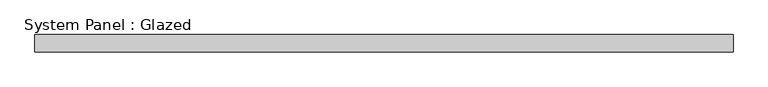
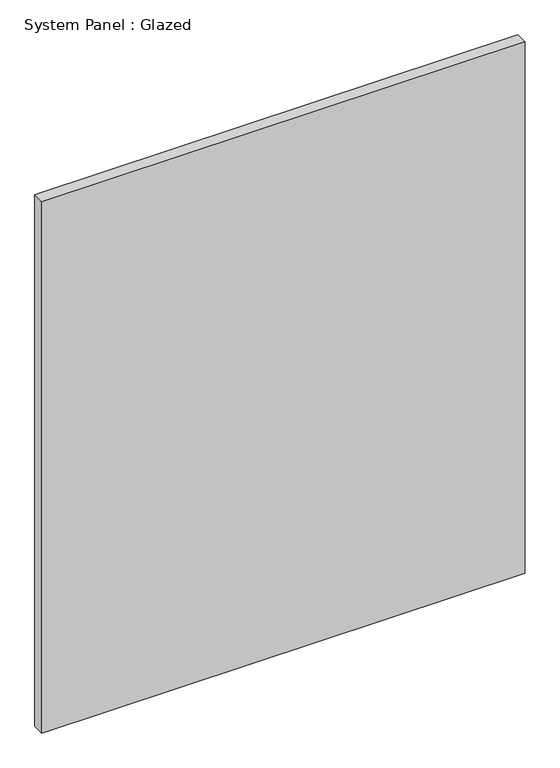
"""IFC4 building model written with IfcOpenShell, lengths in millimetres: plate geometry, System Panel : Glazed."""

from ifc_helpers import new_model, si_unit, origin, origin_with_axes, place, context, project, spatial, polyline, outline, extrude, source, transform, mapped, element, save


def system_panel_glazed_9c96ef9a(model_context):
    return source(origin(), model_context, "Body", "SweptSolid", [
        extrude(outline(polyline([(508.92075, 19.05), (-508.92075, 19.05), (-508.92075, 44.45), (508.92075, 44.45), (508.92075, 19.05)])), origin_with_axes(), (0.0, 0.0, 1.0), 1182.9415),
    ])


if __name__ == "__main__":
    model = new_model("IFC4")
    model_context = context("Model", 3, world=origin())
    ifc_project = project(units=[si_unit("LENGTHUNIT", "METRE", prefix="MILLI")], contexts=[model_context])
    site = spatial("IfcSite", under=ifc_project)
    building = spatial("IfcBuilding", under=site)
    placement = place(None, origin())
    system_panel_glazed_shape = system_panel_glazed_9c96ef9a(model_context)
    element("IfcPlate", 1, ObjectType="System Panel : Glazed", at=placement, inside=building, context=model_context, shape_type="MappedRepresentation", body=[
        mapped(system_panel_glazed_shape, transform((0.0, 0.0, 0.0), x_axis=(1.0, 0.0, 0.0), y_axis=(0.0, 1.0, 0.0), z_axis=(0.0, 0.0, 1.0))),
    ])
    save(model, "model.ifc")

# Revit data of these elements
# Type "System Panel : Glazed"
#   Construction Type Id = "GSP4R"
#   Analytic Construction = "1/8 in Pilkington single glazing"
#   Visual Light Transmittance = 0.9
#   Solar Heat Gain Coefficient = 0.86
#   Heat Transfer Coefficient (U) = 1.18115 BTU/(h·ft²·°F)
#   Define Thermal Properties by = 1
# Element 1 (IfcPlate, "System Panel : Glazed")
#   Materials on its faces: "Glass"
# Materials
#   "Glass": class "Glass", colour RGB 0 128 192, transparency 0.75, Description = "Soda Lime Glass", Cost = 0
